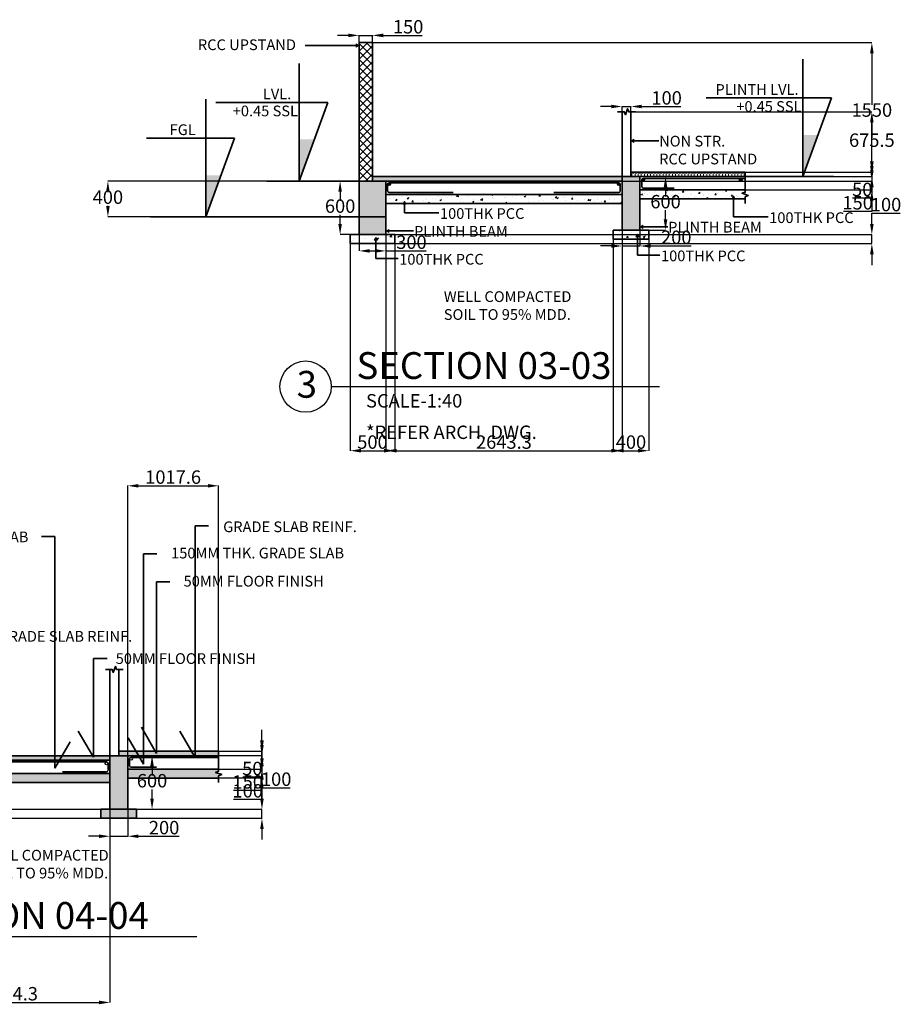
# Model space of a CAD drawing. Units: millimetres. Extents: x -174 to 32373, y 27344 to 53129.
# Tile 6 of 7: x 21438 to 31305, y 27859 to 38879. Entities that reach past the tile are written whole.
import ezdxf

# ---------------------------------------------------------------- set-up
doc = ezdxf.new("R2010")
doc.units = ezdxf.units.MM
doc.header["$LTSCALE"] = 50
for name, color, linetype, lineweight in [('S-ANNO-DIMS', 2, 'Continuous', 18), ('S-ANNO-SYMB', 4, 'Continuous', 25), ('S-ANNO-TEXT', 3, 'Continuous', 18), ('S-DETL', 7, 'Continuous', 35), ('S-PATT', 8, 'Continuous', 13), ('S-REIN', 1, 'Continuous', 25)]:
    doc.layers.add(name, color=color, linetype=linetype, lineweight=lineweight)
doc.styles.get("Standard").update_dxf_attribs({"font": 'arial.ttf'})
doc.dimstyles.new('ISO-25', dxfattribs={"dimtxt": 150, "dimasz": 120, "dimexe": 1.25, "dimexo": 0.625, "dimtad": 1, "dimtih": 1, "dimtoh": 1, "dimdec": 0, "dimtxsty": 'Standard', "dimcen": 2.5, "dimadec": 0, "dimazin": 0, "dimtfac": 1, "dimtdec": 0, "dimtmove": 0, "dimatfit": 3, "dimfxl": 1, "dimarcsym": 0})
pattern_1 = [(0, (0, 0), (0, 34.925), [25.4, -9.525]), (90, (0, 0), (-34.925, 2e-15), [25.4, -9.525])]

# ---------------------------------------------------------------- blocks, each defined once
blk = doc.blocks.new('*D20')
at = {"layer": 'Defpoints', "color": 0, "transparency": 16777216}
for p in [(28179, 36523), (28379, 36523), (28379, 36346)]:
    blk.add_point(p, dxfattribs=at)
at = {"layer": 'S-ANNO-DIMS', "color": 0, "lineweight": -2, "transparency": 16777216}
for p, q in [((28179, 36522), (28179, 36345)), ((28379, 36522), (28379, 36345)), ((28059, 36346), (27939, 36346)), ((28179, 36346), (28379, 36346)), ((28499, 36346), (28954, 36346))]:
    blk.add_line(p, q, dxfattribs=at)
at = {"layer": 'S-ANNO-DIMS', "color": 0, "transparency": 16777216}
for points in [[(28059, 36366), (28059, 36326), (28179, 36346)], [(28499, 36366), (28499, 36326), (28379, 36346)]]:
    blk.add_solid(points, dxfattribs=at)
at = {"layer": 'S-ANNO-DIMS', "color": 0, "transparency": 16777216, "insert": (28786, 36424), "char_height": 150, "attachment_point": 5}
blk.add_mtext('200', dxfattribs=at)
blk = doc.blocks.new('*D21')
at = {"layer": 'Defpoints', "color": 0, "transparency": 16777216}
for p in [(28379, 37123), (28666, 37123), (28379, 36523)]:
    blk.add_point(p, dxfattribs=at)
at = {"layer": 'S-ANNO-DIMS', "color": 0, "lineweight": -2, "transparency": 16777216}
for p, q in [((28380, 37123), (28667, 37123)), ((28666, 37003), (28666, 36900)), ((28666, 36643), (28666, 36746)), ((28380, 36523), (28667, 36523))]:
    blk.add_line(p, q, dxfattribs=at)
at = {"layer": 'S-ANNO-DIMS', "color": 0, "transparency": 16777216}
for points in [[(28646, 37003), (28686, 37003), (28666, 37123)], [(28646, 36643), (28686, 36643), (28666, 36523)]]:
    blk.add_solid(points, dxfattribs=at)
at = {"layer": 'S-ANNO-DIMS', "color": 0, "transparency": 16777216, "insert": (28666, 36823), "char_height": 150, "attachment_point": 5}
blk.add_mtext('600', dxfattribs=at)
blk = doc.blocks.new('*D22')
at = {"layer": 'Defpoints', "color": 0, "transparency": 16777216}
for p in [(25024, 37073), (25536, 37073), (25536, 36473)]:
    blk.add_point(p, dxfattribs=at)
at = {"layer": 'S-ANNO-DIMS', "color": 0, "lineweight": -2, "transparency": 16777216}
for p, q in [((25535, 37073), (25023, 37073)), ((25024, 36953), (25024, 36850)), ((25024, 36593), (25024, 36696)), ((25535, 36473), (25023, 36473))]:
    blk.add_line(p, q, dxfattribs=at)
at = {"layer": 'S-ANNO-DIMS', "color": 0, "transparency": 16777216}
for points in [[(25004, 36953), (25044, 36953), (25024, 37073)], [(25004, 36593), (25044, 36593), (25024, 36473)]]:
    blk.add_solid(points, dxfattribs=at)
at = {"layer": 'S-ANNO-DIMS', "color": 0, "transparency": 16777216, "insert": (25024, 36773), "char_height": 150, "attachment_point": 5}
blk.add_mtext('600', dxfattribs=at)
blk = doc.blocks.new('*D23')
at = {"layer": 'Defpoints', "color": 0, "transparency": 16777216}
for p in [(25236, 36473), (25536, 36473), (25536, 36291)]:
    blk.add_point(p, dxfattribs=at)
at = {"layer": 'S-ANNO-DIMS', "color": 0, "lineweight": -2, "transparency": 16777216}
for p, q in [((25236, 36472), (25236, 36290)), ((25536, 36472), (25536, 36290)), ((25356, 36291), (25416, 36291)), ((25536, 36291), (25988, 36291))]:
    blk.add_line(p, q, dxfattribs=at)
at = {"layer": 'S-ANNO-DIMS', "color": 0, "transparency": 16777216}
for points in [[(25356, 36311), (25356, 36271), (25236, 36291)], [(25416, 36311), (25416, 36271), (25536, 36291)]]:
    blk.add_solid(points, dxfattribs=at)
at = {"layer": 'S-ANNO-DIMS', "color": 0, "transparency": 16777216, "insert": (25822, 36369), "char_height": 150, "attachment_point": 5}
blk.add_mtext('300', dxfattribs=at)
blk = doc.blocks.new('*D24')
at = {"layer": 'Defpoints', "color": 0, "transparency": 16777216}
for p in [(25386, 38703), (25236, 38623), (25386, 38623)]:
    blk.add_point(p, dxfattribs=at)
at = {"layer": 'S-ANNO-DIMS', "color": 0, "lineweight": -2, "transparency": 16777216}
for p, q in [((25116, 38703), (24996, 38703)), ((25236, 38624), (25236, 38704)), ((25236, 38703), (25386, 38703)), ((25386, 38624), (25386, 38704)), ((25506, 38703), (25944, 38703))]:
    blk.add_line(p, q, dxfattribs=at)
at = {"layer": 'S-ANNO-DIMS', "color": 0, "transparency": 16777216}
for points in [[(25116, 38723), (25116, 38683), (25236, 38703)], [(25506, 38723), (25506, 38683), (25386, 38703)]]:
    blk.add_solid(points, dxfattribs=at)
at = {"layer": 'S-ANNO-DIMS', "color": 0, "transparency": 16777216, "insert": (25785, 38780), "char_height": 150, "attachment_point": 5}
blk.add_mtext('150', dxfattribs=at)
blk = doc.blocks.new('*D25')
at = {"layer": 'Defpoints', "color": 0, "transparency": 16777216}
for p in [(28179, 37849), (28279, 37907), (28279, 37849)]:
    blk.add_point(p, dxfattribs=at)
at = {"layer": 'S-ANNO-DIMS', "color": 0, "lineweight": -2, "transparency": 16777216}
for p, q in [((28179, 37849), (28179, 37908)), ((28279, 37849), (28279, 37908)), ((28059, 37907), (27939, 37907)), ((28179, 37907), (28279, 37907)), ((28399, 37907), (28837, 37907))]:
    blk.add_line(p, q, dxfattribs=at)
at = {"layer": 'S-ANNO-DIMS', "color": 0, "transparency": 16777216}
for points in [[(28059, 37927), (28059, 37887), (28179, 37907)], [(28399, 37927), (28399, 37887), (28279, 37907)]]:
    blk.add_solid(points, dxfattribs=at)
at = {"layer": 'S-ANNO-DIMS', "color": 0, "transparency": 16777216, "insert": (28678, 37984), "char_height": 150, "attachment_point": 5}
blk.add_mtext('100', dxfattribs=at)
blk = doc.blocks.new('*D27')
at = {"layer": 'Defpoints', "color": 0, "transparency": 16777216}
for p in [(22447, 30042), (22647, 30042), (22647, 29740)]:
    blk.add_point(p, dxfattribs=at)
at = {"layer": 'S-ANNO-DIMS', "color": 0, "lineweight": -2, "transparency": 16777216}
for p, q in [((22447, 30041), (22447, 29739)), ((22647, 30041), (22647, 29739)), ((22327, 29740), (22207, 29740)), ((22447, 29740), (22647, 29740)), ((22767, 29740), (23221, 29740))]:
    blk.add_line(p, q, dxfattribs=at)
at = {"layer": 'S-ANNO-DIMS', "color": 0, "transparency": 16777216}
for points in [[(22327, 29760), (22327, 29720), (22447, 29740)], [(22767, 29760), (22767, 29720), (22647, 29740)]]:
    blk.add_solid(points, dxfattribs=at)
at = {"layer": 'S-ANNO-DIMS', "color": 0, "transparency": 16777216, "insert": (23054, 29817), "char_height": 150, "attachment_point": 5}
blk.add_mtext('200', dxfattribs=at)
blk = doc.blocks.new('*D29')
at = {"layer": 'Defpoints', "color": 0, "transparency": 16777216}
for p in [(22647, 30642), (22647, 30042), (22919, 30042)]:
    blk.add_point(p, dxfattribs=at)
at = {"layer": 'S-ANNO-DIMS', "color": 0, "lineweight": -2, "transparency": 16777216}
for p, q in [((22647, 30642), (22921, 30642)), ((22919, 30522), (22919, 30419)), ((22919, 30162), (22919, 30265)), ((22647, 30042), (22921, 30042))]:
    blk.add_line(p, q, dxfattribs=at)
at = {"layer": 'S-ANNO-DIMS', "color": 0, "transparency": 16777216}
for points in [[(22899, 30522), (22939, 30522), (22919, 30642)], [(22899, 30162), (22939, 30162), (22919, 30042)]]:
    blk.add_solid(points, dxfattribs=at)
at = {"layer": 'S-ANNO-DIMS', "color": 0, "transparency": 16777216, "insert": (22919, 30342), "char_height": 150, "attachment_point": 5}
blk.add_mtext('600', dxfattribs=at)
blk = doc.blocks.new('SECTION-MARK')
blk.add_line((575, 287), (4248, 287))
blk.add_circle((287, 287), 287)
blk = doc.blocks.new('*D76')
at = {"layer": 'Defpoints', "color": 0, "transparency": 16777216}
for p in [(22425, 37073), (25236, 37073), (25536, 36673)]:
    blk.add_point(p, dxfattribs=at)
at = {"layer": 'S-ANNO-DIMS', "color": 0, "lineweight": -2, "transparency": 16777216}
for p, q in [((25235, 37073), (22424, 37073)), ((22425, 36953), (22425, 36950)), ((22425, 36793), (22425, 36796)), ((25535, 36673), (22424, 36673))]:
    blk.add_line(p, q, dxfattribs=at)
at = {"layer": 'S-ANNO-DIMS', "color": 0, "transparency": 16777216}
for points in [[(22405, 36953), (22445, 36953), (22425, 37073)], [(22405, 36793), (22445, 36793), (22425, 36673)]]:
    blk.add_solid(points, dxfattribs=at)
at = {"layer": 'S-ANNO-DIMS', "color": 0, "transparency": 16777216, "insert": (22425, 36873), "char_height": 150, "attachment_point": 5}
blk.add_mtext('400', dxfattribs=at)
blk = doc.blocks.new('*D77')
at = {"layer": 'Defpoints', "color": 0, "transparency": 16777216}
for p in [(25386, 38623), (30975, 38623), (25386, 37073)]:
    blk.add_point(p, dxfattribs=at)
at = {"layer": 'S-ANNO-DIMS', "color": 0, "lineweight": -2, "transparency": 16777216}
for p, q in [((25386, 38623), (30976, 38623)), ((30975, 38503), (30975, 37925)), ((30975, 37193), (30975, 37771)), ((25386, 37073), (30976, 37073))]:
    blk.add_line(p, q, dxfattribs=at)
at = {"layer": 'S-ANNO-DIMS', "color": 0, "transparency": 16777216}
for points in [[(30955, 38503), (30995, 38503), (30975, 38623)], [(30955, 37193), (30995, 37193), (30975, 37073)]]:
    blk.add_solid(points, dxfattribs=at)
at = {"layer": 'S-ANNO-DIMS', "color": 0, "transparency": 16777216, "insert": (30975, 37848), "char_height": 150, "attachment_point": 5}
blk.add_mtext('1550', dxfattribs=at)
blk = doc.blocks.new('*D78')
at = {"layer": 'Defpoints', "color": 0, "transparency": 16777216}
for p in [(28179, 36523), (25536, 36473), (28179, 34055)]:
    blk.add_point(p, dxfattribs=at)
at = {"layer": 'S-ANNO-DIMS', "color": 0, "lineweight": -2, "transparency": 16777216}
for p, q in [((28179, 36522), (28179, 34054)), ((25536, 36472), (25536, 34054)), ((25656, 34055), (28059, 34055))]:
    blk.add_line(p, q, dxfattribs=at)
at = {"layer": 'S-ANNO-DIMS', "color": 0, "transparency": 16777216}
for points in [[(25656, 34075), (25656, 34035), (25536, 34055)], [(28059, 34075), (28059, 34035), (28179, 34055)]]:
    blk.add_solid(points, dxfattribs=at)
at = {"layer": 'S-ANNO-DIMS', "color": 0, "transparency": 16777216, "insert": (26857, 34132), "char_height": 150, "attachment_point": 5}
blk.add_mtext('2643.3', dxfattribs=at)
blk = doc.blocks.new('*D79')
at = {"layer": 'Defpoints', "color": 0, "transparency": 16777216}
for p in [(29557, 37173), (28379, 37123), (30975, 37123)]:
    blk.add_point(p, dxfattribs=at)
at = {"layer": 'S-ANNO-DIMS', "color": 0, "lineweight": -2, "transparency": 16777216}
for p, q in [((30975, 37293), (30975, 37413)), ((29558, 37173), (30976, 37173)), ((30975, 37173), (30975, 37123)), ((28380, 37123), (30976, 37123)), ((30975, 37003), (30975, 36883)), ((30975, 36883), (30760, 36883))]:
    blk.add_line(p, q, dxfattribs=at)
at = {"layer": 'S-ANNO-DIMS', "color": 0, "transparency": 16777216}
for points in [[(30955, 37293), (30995, 37293), (30975, 37173)], [(30955, 37003), (30995, 37003), (30975, 37123)]]:
    blk.add_solid(points, dxfattribs=at)
at = {"layer": 'S-ANNO-DIMS', "color": 0, "transparency": 16777216, "insert": (30867, 36960), "char_height": 150, "attachment_point": 5}
blk.add_mtext('50', dxfattribs=at)
blk = doc.blocks.new('*D80')
at = {"layer": 'Defpoints', "color": 0, "transparency": 16777216}
for p in [(28379, 37123), (29557, 36973), (30975, 36973)]:
    blk.add_point(p, dxfattribs=at)
at = {"layer": 'S-ANNO-DIMS', "color": 0, "lineweight": -2, "transparency": 16777216}
for p, q in [((30975, 37243), (30975, 37363)), ((28380, 37123), (30976, 37123)), ((30975, 37123), (30975, 36973)), ((29558, 36973), (30976, 36973)), ((30975, 36853), (30975, 36733)), ((30975, 36733), (30658, 36733))]:
    blk.add_line(p, q, dxfattribs=at)
at = {"layer": 'S-ANNO-DIMS', "color": 0, "transparency": 16777216}
for points in [[(30955, 37243), (30995, 37243), (30975, 37123)], [(30955, 36853), (30995, 36853), (30975, 36973)]]:
    blk.add_solid(points, dxfattribs=at)
at = {"layer": 'S-ANNO-DIMS', "color": 0, "transparency": 16777216, "insert": (30816, 36810), "char_height": 150, "attachment_point": 5}
blk.add_mtext('150', dxfattribs=at)
blk = doc.blocks.new('*D81')
at = {"layer": 'Defpoints', "color": 0, "transparency": 16777216}
for p in [(28279, 37849), (30975, 37849), (28279, 37173)]:
    blk.add_point(p, dxfattribs=at)
at = {"layer": 'S-ANNO-DIMS', "color": 0, "lineweight": -2, "transparency": 16777216}
for p, q in [((28280, 37849), (30976, 37849)), ((30975, 37729), (30975, 37588)), ((30975, 37293), (30975, 37434)), ((28280, 37173), (30976, 37173))]:
    blk.add_line(p, q, dxfattribs=at)
at = {"layer": 'S-ANNO-DIMS', "color": 0, "transparency": 16777216}
for points in [[(30955, 37729), (30995, 37729), (30975, 37849)], [(30955, 37293), (30995, 37293), (30975, 37173)]]:
    blk.add_solid(points, dxfattribs=at)
at = {"layer": 'S-ANNO-DIMS', "color": 0, "transparency": 16777216, "insert": (30975, 37511), "char_height": 150, "attachment_point": 5}
blk.add_mtext('675.5', dxfattribs=at)
blk = doc.blocks.new('*D82')
at = {"layer": 'Defpoints', "color": 0, "transparency": 16777216}
for p in [(25136, 36373), (25636, 36373), (25636, 34055)]:
    blk.add_point(p, dxfattribs=at)
at = {"layer": 'S-ANNO-DIMS', "color": 0, "lineweight": -2, "transparency": 16777216}
for p, q in [((25136, 36372), (25136, 34054)), ((25636, 36372), (25636, 34054)), ((25256, 34055), (25516, 34055))]:
    blk.add_line(p, q, dxfattribs=at)
at = {"layer": 'S-ANNO-DIMS', "color": 0, "transparency": 16777216}
for points in [[(25256, 34075), (25256, 34035), (25136, 34055)], [(25516, 34075), (25516, 34035), (25636, 34055)]]:
    blk.add_solid(points, dxfattribs=at)
at = {"layer": 'S-ANNO-DIMS', "color": 0, "transparency": 16777216, "insert": (25386, 34132), "char_height": 150, "attachment_point": 5}
blk.add_mtext('500', dxfattribs=at)
blk = doc.blocks.new('*D83')
at = {"layer": 'Defpoints', "color": 0, "transparency": 16777216}
for p in [(28079, 36423), (28479, 36423), (28479, 34055)]:
    blk.add_point(p, dxfattribs=at)
at = {"layer": 'S-ANNO-DIMS', "color": 0, "lineweight": -2, "transparency": 16777216}
for p, q in [((28079, 36422), (28079, 34054)), ((28479, 36422), (28479, 34054)), ((28199, 34055), (28359, 34055))]:
    blk.add_line(p, q, dxfattribs=at)
at = {"layer": 'S-ANNO-DIMS', "color": 0, "transparency": 16777216}
for points in [[(28199, 34075), (28199, 34035), (28079, 34055)], [(28359, 34075), (28359, 34035), (28479, 34055)]]:
    blk.add_solid(points, dxfattribs=at)
at = {"layer": 'S-ANNO-DIMS', "color": 0, "transparency": 16777216, "insert": (28279, 34132), "char_height": 150, "attachment_point": 5}
blk.add_mtext('400', dxfattribs=at)
blk = doc.blocks.new('*D84')
at = {"layer": 'Defpoints', "color": 0, "transparency": 16777216}
for p in [(25636, 36473), (25636, 36373), (30975, 36473)]:
    blk.add_point(p, dxfattribs=at)
at = {"layer": 'S-ANNO-DIMS', "color": 0, "lineweight": -2, "transparency": 16777216}
for p, q in [((30975, 36593), (30975, 36713)), ((30975, 36713), (31293, 36713)), ((25636, 36473), (30976, 36473)), ((25636, 36373), (30976, 36373)), ((30975, 36373), (30975, 36473)), ((30975, 36253), (30975, 36133))]:
    blk.add_line(p, q, dxfattribs=at)
at = {"layer": 'S-ANNO-DIMS', "color": 0, "transparency": 16777216}
for points in [[(30955, 36593), (30995, 36593), (30975, 36473)], [(30955, 36253), (30995, 36253), (30975, 36373)]]:
    blk.add_solid(points, dxfattribs=at)
at = {"layer": 'S-ANNO-DIMS', "color": 0, "transparency": 16777216, "insert": (31134, 36790), "char_height": 150, "attachment_point": 5}
blk.add_mtext('100', dxfattribs=at)
blk = doc.blocks.new('*D85')
at = {"layer": 'Defpoints', "color": 0, "transparency": 16777216}
for p in [(20212, 30042), (22447, 30042), (22447, 27880)]:
    blk.add_point(p, dxfattribs=at)
at = {"layer": 'S-ANNO-DIMS', "color": 0, "lineweight": -2, "transparency": 16777216}
for p, q in [((20212, 30041), (20212, 27879)), ((22447, 30041), (22447, 27879)), ((20332, 27880), (22327, 27880))]:
    blk.add_line(p, q, dxfattribs=at)
at = {"layer": 'S-ANNO-DIMS', "color": 0, "transparency": 16777216}
for points in [[(20332, 27900), (20332, 27860), (20212, 27880)], [(22327, 27900), (22327, 27860), (22447, 27880)]]:
    blk.add_solid(points, dxfattribs=at)
at = {"layer": 'S-ANNO-DIMS', "color": 0, "transparency": 16777216, "insert": (21330, 27958), "char_height": 150, "attachment_point": 5}
blk.add_mtext('2234.3', dxfattribs=at)
blk = doc.blocks.new('*D86')
at = {"layer": 'Defpoints', "color": 0, "transparency": 16777216}
for p in [(22647, 30642), (23664, 30692), (24149, 30642)]:
    blk.add_point(p, dxfattribs=at)
at = {"layer": 'S-ANNO-DIMS', "color": 0, "lineweight": -2, "transparency": 16777216}
for p, q in [((24149, 30812), (24149, 30932)), ((22647, 30642), (24150, 30642)), ((23665, 30692), (24150, 30692)), ((24149, 30692), (24149, 30642)), ((24149, 30522), (24149, 30402)), ((24149, 30402), (23934, 30402))]:
    blk.add_line(p, q, dxfattribs=at)
at = {"layer": 'S-ANNO-DIMS', "color": 0, "transparency": 16777216}
for points in [[(24129, 30812), (24169, 30812), (24149, 30692)], [(24129, 30522), (24169, 30522), (24149, 30642)]]:
    blk.add_solid(points, dxfattribs=at)
at = {"layer": 'S-ANNO-DIMS', "color": 0, "transparency": 16777216, "insert": (24041, 30479), "char_height": 150, "attachment_point": 5}
blk.add_mtext('50', dxfattribs=at)
blk = doc.blocks.new('*D87')
at = {"layer": 'Defpoints', "color": 0, "transparency": 16777216}
for p in [(22647, 30642), (23664, 30492), (24149, 30492)]:
    blk.add_point(p, dxfattribs=at)
at = {"layer": 'S-ANNO-DIMS', "color": 0, "lineweight": -2, "transparency": 16777216}
for p, q in [((24149, 30762), (24149, 30882)), ((22647, 30642), (24150, 30642)), ((24149, 30642), (24149, 30492)), ((23665, 30492), (24150, 30492)), ((24149, 30372), (24149, 30252)), ((24149, 30252), (23831, 30252))]:
    blk.add_line(p, q, dxfattribs=at)
at = {"layer": 'S-ANNO-DIMS', "color": 0, "transparency": 16777216}
for points in [[(24129, 30762), (24169, 30762), (24149, 30642)], [(24129, 30372), (24169, 30372), (24149, 30492)]]:
    blk.add_solid(points, dxfattribs=at)
at = {"layer": 'S-ANNO-DIMS', "color": 0, "transparency": 16777216, "insert": (23990, 30329), "char_height": 150, "attachment_point": 5}
blk.add_mtext('150', dxfattribs=at)
blk = doc.blocks.new('*D88')
at = {"layer": 'Defpoints', "color": 0, "transparency": 16777216}
for p in [(23664, 30492), (23664, 30392), (24149, 30392)]:
    blk.add_point(p, dxfattribs=at)
at = {"layer": 'S-ANNO-DIMS', "color": 0, "lineweight": -2, "transparency": 16777216}
for p, q in [((24149, 30612), (24149, 30732)), ((23665, 30492), (24150, 30492)), ((24149, 30492), (24149, 30392)), ((23665, 30392), (24150, 30392)), ((24149, 30272), (24149, 30152)), ((24149, 30152), (23831, 30152))]:
    blk.add_line(p, q, dxfattribs=at)
at = {"layer": 'S-ANNO-DIMS', "color": 0, "transparency": 16777216}
for points in [[(24129, 30612), (24169, 30612), (24149, 30492)], [(24129, 30272), (24169, 30272), (24149, 30392)]]:
    blk.add_solid(points, dxfattribs=at)
at = {"layer": 'S-ANNO-DIMS', "color": 0, "transparency": 16777216, "insert": (23990, 30229), "char_height": 150, "attachment_point": 5}
blk.add_mtext('100', dxfattribs=at)
blk = doc.blocks.new('*D90')
at = {"layer": 'Defpoints', "color": 0, "transparency": 16777216}
for p in [(23664, 33662), (22647, 30642), (23664, 30692)]:
    blk.add_point(p, dxfattribs=at)
at = {"layer": 'S-ANNO-DIMS', "color": 0, "lineweight": -2, "transparency": 16777216}
for p, q in [((22647, 30642), (22647, 33664)), ((22767, 33662), (23544, 33662)), ((23664, 30692), (23664, 33664))]:
    blk.add_line(p, q, dxfattribs=at)
at = {"layer": 'S-ANNO-DIMS', "color": 0, "transparency": 16777216}
for points in [[(22767, 33682), (22767, 33642), (22647, 33662)], [(23544, 33682), (23544, 33642), (23664, 33662)]]:
    blk.add_solid(points, dxfattribs=at)
at = {"layer": 'S-ANNO-DIMS', "color": 0, "transparency": 16777216, "insert": (23155, 33740), "char_height": 150, "attachment_point": 5}
blk.add_mtext('1017.6', dxfattribs=at)
blk = doc.blocks.new('*D92')
at = {"layer": 'Defpoints', "color": 0, "transparency": 16777216}
for p in [(20312, 30042), (24149, 30042), (20312, 29942)]:
    blk.add_point(p, dxfattribs=at)
at = {"layer": 'S-ANNO-DIMS', "color": 0, "lineweight": -2, "transparency": 16777216}
for p, q in [((24149, 30162), (24149, 30282)), ((24149, 30282), (24466, 30282)), ((20313, 30042), (24150, 30042)), ((24149, 29942), (24149, 30042)), ((20313, 29942), (24150, 29942)), ((24149, 29822), (24149, 29702))]:
    blk.add_line(p, q, dxfattribs=at)
at = {"layer": 'S-ANNO-DIMS', "color": 0, "transparency": 16777216}
for points in [[(24129, 30162), (24169, 30162), (24149, 30042)], [(24129, 29822), (24169, 29822), (24149, 29942)]]:
    blk.add_solid(points, dxfattribs=at)
at = {"layer": 'S-ANNO-DIMS', "color": 0, "transparency": 16777216, "insert": (24308, 30359), "char_height": 150, "attachment_point": 5}
blk.add_mtext('100', dxfattribs=at)

msp = doc.modelspace()

# ---------------------------------------------------------------- hatches: boundary and pattern name
at = {"layer": 'S-ANNO-SYMB'}
h = msp.add_hatch(color=256, dxfattribs=at)
h.dxf.hatch_style = 1
h.paths.add_polyline_path([(30201.87, 37123.04), (30371.08, 37587.96), (30201.87, 37587.96)])
h = msp.add_hatch(color=256, dxfattribs=at)
h.dxf.hatch_style = 1
h.paths.add_polyline_path([(24566.02, 37073.04), (24735.24, 37537.96), (24566.02, 37537.96)])
h = msp.add_hatch(color=256, dxfattribs=at)
h.dxf.hatch_style = 1
h.paths.add_polyline_path([(23522.69, 36673.04), (23691.91, 37137.96), (23522.69, 37137.96)])
at = {"layer": 'S-ANNO-TEXT'}
h = msp.add_hatch(color=256, dxfattribs=at)
h.dxf.hatch_style = 1
h.paths.add_polyline_path([(25204.09, 38607.16), (25204.09, 38570.5), (25235.84, 38588.83)])
h = msp.add_hatch(color=256, dxfattribs=at)
h.dxf.hatch_style = 1
h.paths.add_polyline_path([(28279.14, 37523.37), (28310.89, 37505.04), (28310.89, 37541.71)])
h = msp.add_hatch(color=256, dxfattribs=at)
h.dxf.hatch_style = 1
h.paths.add_polyline_path([(25571.7, 37053.04, 0.40886497), (25555.84, 37037.19, 0.99539446), (25587.26, 37037.33, 0.41151206)])
h = msp.add_hatch(color=256, dxfattribs=at)
h.dxf.hatch_style = 1
h.paths.add_polyline_path([(28159.14, 37037.33, 1), (28127.72, 37037.33, 1)])
h = msp.add_hatch(color=256, dxfattribs=at)
h.dxf.hatch_style = 1
h.paths.add_polyline_path([(28430.56, 37087.33, 1), (28399.14, 37087.33, 1)])
h = msp.add_hatch(color=256, dxfattribs=at)
h.dxf.hatch_style = 1
h.paths.add_polyline_path([(29522.57, 37087.33, 1), (29491.15, 37087.33, 1)])
h = msp.add_hatch(color=256, dxfattribs=at)
h.dxf.hatch_style = 1
h.paths.add_polyline_path([(25743.42, 36845.8), (25725.08, 36814.04), (25761.75, 36814.04)])
h = msp.add_hatch(color=256, dxfattribs=at)
h.dxf.hatch_style = 1
h.paths.add_polyline_path([(29427.68, 36907.17), (29409.34, 36875.42), (29446.01, 36875.42)])
h = msp.add_hatch(color=256, dxfattribs=at)
h.dxf.hatch_style = 1
h.paths.add_polyline_path([(25535.84, 36513.92), (25567.6, 36495.59), (25567.6, 36532.25)])
h = msp.add_hatch(color=256, dxfattribs=at)
h.dxf.hatch_style = 1
h.paths.add_polyline_path([(28352.38, 36479.44), (28334.05, 36447.69), (28370.71, 36447.69)])
h = msp.add_hatch(color=256, dxfattribs=at)
h.dxf.hatch_style = 1
h.paths.add_polyline_path([(28379.14, 36560.36), (28410.89, 36542.03), (28410.89, 36578.69)])
h = msp.add_hatch(color=256, dxfattribs=at)
h.dxf.hatch_style = 1
h.paths.add_polyline_path([(25422.3, 36441.56), (25403.97, 36409.81), (25440.63, 36409.81)])
at = {"layer": 'S-PATT'}
h = msp.add_hatch(dxfattribs=at)
h.set_pattern_fill('ANSI37', color=256, scale=20)
h.paths.add_polyline_path([(25235.84, 37073.04), (25385.84, 37073.04), (25385.84, 38623.04), (25235.84, 38623.04)])
h = msp.add_hatch(dxfattribs=at)
h.set_pattern_fill('ANGLE', color=256, scale=5)
h.set_pattern_definition(pattern_1)
h.paths.add_polyline_path([(29557.2, 37123.04), (29557.2, 37173.04), (28279.14, 37173.04), (28279.14, 37123.04), (28379.14, 37123.04)])
h = msp.add_hatch(color=256, dxfattribs=at)
h.dxf.hatch_style = 1
h.paths.add_polyline_path([(25535.84, 37073.04), (25235.84, 37073.04), (25235.84, 36473.04), (25535.84, 36473.04)])
h = msp.add_hatch(dxfattribs=at)
h.set_pattern_fill('ANGLE', color=256, scale=5)
h.set_pattern_definition(pattern_1)
h.paths.add_polyline_path([(28179.14, 37073.04), (28179.14, 37123.04), (25385.84, 37123.04), (25385.84, 37073.04), (25535.84, 37073.04)])
h = msp.add_hatch(color=256, dxfattribs=at)
h.dxf.hatch_style = 1
h.paths.add_polyline_path([(28179.14, 36523.04), (28379.14, 36523.04), (28379.14, 37123.04), (28179.14, 37123.04)])
h = msp.add_hatch(dxfattribs=at)
h.set_pattern_fill('AR-CONC', color=256)
h.paths.add_polyline_path([(28179.14, 36923.04), (25535.84, 36923.04), (25535.84, 36823.04), (28179.14, 36823.04)])
h = msp.add_hatch(dxfattribs=at)
h.set_pattern_fill('AR-CONC', color=256)
h.paths.add_polyline_path([(28379.14, 36973.04), (28379.14, 36873.04), (29557.2, 36873.04), (29557.2, 36898.04), (29591.54, 36910.54), (29522.86, 36935.54), (29557.2, 36948.04), (29557.2, 36973.04)])
h = msp.add_hatch(dxfattribs=at)
h.set_pattern_fill('AR-CONC', color=256)
h.paths.add_polyline_path([(28479.14, 36523.04), (28379.14, 36523.04), (28179.14, 36523.04), (28079.14, 36523.04), (28079.14, 36423.04), (28479.14, 36423.04)])
h = msp.add_hatch(dxfattribs=at)
h.set_pattern_fill('AR-CONC', color=256)
h.paths.add_polyline_path([(25635.84, 36473.04), (25535.84, 36473.04), (25235.84, 36473.04), (25135.84, 36473.04), (25135.84, 36373.04), (25635.84, 36373.04)])
h = msp.add_hatch(dxfattribs=at)
h.set_pattern_fill('ANGLE', color=256, scale=5)
h.set_pattern_definition([(0, (-5178.336, 733.413), (0, 34.925), [25.4, -9.525]), (90, (-5178.336, 733.413), (-34.925, 2e-15), [25.4, -9.525])])
h.paths.add_polyline_path([(22446.68, 30591.75), (22446.68, 30641.75), (20212.39, 30641.75), (20212.39, 30591.75)])
h.paths.add_polyline_path([(20012.39, 30641.75), (20112.39, 30641.75), (20112.39, 30691.75), (19005.68, 30691.75), (19005.68, 30641.75)])
h.paths.add_polyline_path([(22546.68, 30691.75), (22546.68, 30641.75), (22646.68, 30641.75), (23664.24, 30641.75), (23664.24, 30691.75)])
h = msp.add_hatch(color=256, dxfattribs=at)
h.dxf.hatch_style = 1
h.paths.add_polyline_path([(20212.39, 30641.75), (20012.39, 30641.75), (20012.39, 30041.75), (20212.39, 30041.75)])
h.paths.add_polyline_path([(22646.68, 30641.75), (22446.68, 30641.75), (22446.68, 30041.75), (22646.68, 30041.75)])
h = msp.add_hatch(dxfattribs=at)
h.set_pattern_fill('AR-CONC', color=256)
h.set_pattern_definition([(50, (-5178.34, 733.41), (182.18467, -15.9391), [19.05, -209.55]), (355, (-5178.34, 733.41), (-35.2434, 191.05685), [15.24, -167.6406]), (100.45144, (-5163.15, 732.09), (146.94125, 175.11775), [16.19, -178.09024]), (46.1842, (-5178.34, 784.21), (271.079, -42.0423), [28.575, -314.325]), (96.63556, (-5155.75, 780.7), (237.4041, 247.4261), [24.285, -267.1356]), (351.18415, (-5178.34, 784.2), (237.4041, 247.4261), [22.86, -251.4597]), (21, (-5152.94, 771.51), (151.6144, -102.2652), [19.05, -209.55]), (326, (-5152.94, 771.51), (61.802, 184.188), [15.24, -167.64]), (71.45144, (-5140.3, 762.99), (213.4164, 81.9228), [16.19, -178.0899]), (37.5, (-5178.336, 733.413), (3.0886, 84.55504), [0, -165.608, 0, -170.18, 0, -168.275]), (7.5, (-5178.34, 733.41), (66.81966, 100.18057), [0, -97.028, 0, -161.798, 0, -64.135]), (327.5, (-5234.98, 733.41), (135.5906, -5.72874), [0, -63.5, 0, -198.12, 0, -262.89]), (317.5, (-5260.38, 733.41), (148.12918, 25.4265), [0, -82.55, 0, -131.572, 0, -186.69])])
h.paths.add_polyline_path([(20312.39, 29941.75), (20312.39, 30041.75), (20212.39, 30041.75), (20012.39, 30041.75), (19912.39, 30041.75), (19912.39, 29941.75)])
h.paths.add_polyline_path([(22746.68, 29941.75), (22746.68, 30041.75), (22646.68, 30041.75), (22446.68, 30041.75), (22346.68, 30041.75), (22346.68, 29941.75)])
h.paths.add_polyline_path([(22446.68, 30341.75), (22446.68, 30441.75), (20212.39, 30441.75), (20212.39, 30341.75)])
h.paths.add_polyline_path([(23664.24, 30391.75), (23664.24, 30441.75), (23629.9, 30454.25), (23664.24, 30466.75), (23664.24, 30491.75), (22646.68, 30491.75), (22646.68, 30391.75)])
h.paths.add_polyline_path([(20012.39, 30391.75), (20012.39, 30491.75), (19005.68, 30491.75), (19005.68, 30441.75), (19040.02, 30429.25), (19005.68, 30416.75), (19005.68, 30391.75)])

# ---------------------------------------------------------------- linework, layer by layer
at = {"layer": 'S-ANNO-TEXT'}
for points in [[(25235.84, 38588.83), (25204.09, 38570.5), (25204.09, 38607.16)], [(28279.14, 37523.37), (28310.89, 37505.04), (28310.89, 37541.71)], [(25743.42, 36845.8), (25725.08, 36814.04), (25761.75, 36814.04)], [(29427.68, 36907.17), (29409.34, 36875.42), (29446.01, 36875.42)], [(25535.84, 36513.92), (25567.6, 36495.59), (25567.6, 36532.25)], [(28352.38, 36479.44), (28334.05, 36447.69), (28370.71, 36447.69)], [(28379.14, 36560.36), (28410.89, 36542.03), (28410.89, 36578.69)], [(25422.3, 36441.56), (25403.97, 36409.81), (25440.63, 36409.81)]]:
    msp.add_lwpolyline(points, close=True, dxfattribs=at)
at = {"layer": 'S-DETL'}
for p, q in [((25204.09, 38588.83), (24631.33, 38588.83)), ((25235.84, 38623.04), (25235.84, 37073.04)), ((25235.84, 38623.04), (25385.84, 38623.04)), ((25385.84, 38623.04), (25385.84, 37073.04)), ((24566.02, 37073.04), (24566.02, 38388.54)), ((30201.87, 37123.04), (30201.87, 38438.54)), ((23522.69, 36673.04), (23522.69, 37988.54)), ((24886.09, 37952.42), (23633.71, 37952.42)), ((24566.02, 37073.04), (24886.09, 37952.42)), ((30521.93, 38002.42), (29121.86, 38002.42)), ((30201.87, 37123.04), (30521.93, 38002.42)), ((28179.14, 37123.04), (28179.14, 37848.58)), ((28279.14, 37123.04), (28279.14, 37848.58)), ((23842.76, 37552.42), (22855.16, 37552.42)), ((23522.69, 36673.04), (23842.76, 37552.42)), ((28310.89, 37523.37), (28590.28, 37523.37)), ((28279.14, 37173.04), (29557.2, 37173.04)), ((29557.2, 37023.04), (29557.2, 37173.04)), ((25535.84, 37073.04), (24201.98, 37073.04)), ((25235.84, 37073.04), (25235.84, 36473.04)), ((28179.14, 37123.04), (25385.84, 37123.04)), ((28179.14, 37073.04), (25535.84, 37073.04)), ((25535.84, 36473.04), (25535.84, 37073.04)), ((25555.84, 36959.04), (25555.84, 37037.04)), ((28143.14, 37053.04), (25571.84, 37053.04)), ((28159.14, 36959.04), (28159.14, 37037.04)), ((28179.14, 37123.04), (28379.14, 37123.04)), ((28179.14, 36523.04), (28179.14, 37123.04)), ((28379.14, 37123.04), (28379.14, 36523.04)), ((28379.14, 37123.04), (30545.25, 37123.04)), ((28399.14, 37087.04), (28399.14, 37009.04)), ((28415.14, 37103.04), (29557.2, 37103.04)), ((28179.14, 36923.04), (25535.84, 36923.04)), ((26287.99, 36943.04), (25571.84, 36943.04)), ((28143.14, 36943.04), (27415.25, 36943.04)), ((28379.14, 36973.04), (29557.2, 36973.04)), ((28415.14, 36993.04), (28761.4, 36993.04)), ((28179.14, 36823.04), (25535.84, 36823.04)), ((25743.42, 36814.04), (25743.42, 36716.53)), ((28379.14, 36873.04), (29557.2, 36873.04)), ((29427.68, 36875.42), (29427.68, 36670.52)), ((25743.42, 36716.53), (26128.56, 36716.53)), ((25535.84, 36673.04), (22901.76, 36673.04)), ((29427.68, 36670.52), (29812.82, 36670.52)), ((25567.6, 36513.92), (25846.98, 36513.92)), ((28079.14, 36423.04), (28079.14, 36523.04)), ((28079.14, 36523.04), (28179.14, 36523.04)), ((28379.14, 36523.04), (28179.14, 36523.04)), ((28379.14, 36523.04), (28479.14, 36523.04)), ((28410.89, 36560.36), (28690.28, 36560.36)), ((28479.14, 36523.04), (28479.14, 36423.04)), ((25135.84, 36373.04), (25135.84, 36473.04)), ((25135.84, 36473.04), (25235.84, 36473.04)), ((25635.84, 36373.04), (25135.84, 36373.04)), ((25235.84, 36473.04), (25535.84, 36473.04)), ((25422.3, 36409.81), (25422.3, 36204.9)), ((25535.84, 36473.04), (25635.84, 36473.04)), ((25635.84, 36473.04), (25635.84, 36373.04)), ((28479.14, 36423.04), (28079.14, 36423.04)), ((28352.38, 36447.69), (28352.38, 36242.79)), ((25422.3, 36204.9), (25672.31, 36204.9)), ((28352.38, 36242.79), (28602.39, 36242.79)), ((23400.14, 30621.75), (23400.14, 33212.37)), ((23400.14, 33212.37), (23550.45, 33212.37)), ((21831.64, 33093.15), (21681.33, 33093.15)), ((21831.64, 30502.53), (21831.64, 33093.15)), ((22822.41, 30548.08), (22822.41, 32901)), ((22822.41, 32901), (22972.72, 32901)), ((22969.54, 30667.42), (22969.54, 32585.77)), ((22969.54, 32585.77), (23119.85, 32585.77)), ((22263.68, 30623.34), (22263.68, 31727.65)), ((22263.68, 31727.65), (22415.84, 31727.65)), ((22446.68, 30641.75), (22446.68, 31607.24)), ((22546.68, 30641.75), (22546.68, 31607.24)), ((22263.68, 30623.34), (22093.67, 30917.81)), ((22969.54, 30667.42), (22799.53, 30961.89)), ((23400.14, 30621.75), (23230.12, 30916.22)), ((21831.64, 30502.53), (22001.66, 30797)), ((22822.41, 30548.08), (22652.4, 30842.55)), ((20212.39, 30641.75), (22446.68, 30641.75)), ((22446.68, 30641.75), (22646.68, 30641.75)), ((22446.68, 30041.75), (22446.68, 30641.75)), ((22546.68, 30641.75), (22546.68, 30691.75)), ((22546.68, 30691.75), (23664.24, 30691.75)), ((22646.68, 30641.75), (22646.68, 30041.75)), ((22646.68, 30641.75), (23664.24, 30641.75)), ((23664.24, 30691.75), (23664.24, 30491.75)), ((20212.39, 30591.75), (22446.68, 30591.75)), ((20248.39, 30571.75), (22410.68, 30571.75)), ((22426.68, 30477.75), (22426.68, 30555.75)), ((22666.68, 30605.75), (22666.68, 30527.75)), ((22682.68, 30621.75), (23664.24, 30621.75)), ((20212.39, 30441.75), (22446.68, 30441.75)), ((21918.54, 30461.75), (22410.68, 30461.75)), ((22646.68, 30491.75), (23664.24, 30491.75)), ((22682.68, 30511.75), (22968.77, 30511.75)), ((20212.39, 30341.75), (22446.68, 30341.75)), ((22646.68, 30391.75), (23664.24, 30391.75)), ((22346.68, 29941.75), (22346.68, 30041.75)), ((22346.68, 30041.75), (22446.68, 30041.75)), ((22646.68, 30041.75), (22446.68, 30041.75)), ((22646.68, 30041.75), (22746.68, 30041.75)), ((22746.68, 30041.75), (22746.68, 29941.75)), ((22746.68, 29941.75), (22346.68, 29941.75))]:
    msp.add_line(p, q, dxfattribs=at)
for points in [[(28129.14, 37848.58), (28204.14, 37848.58), (28216.64, 37814.24), (28241.64, 37882.93), (28254.14, 37848.58), (28329.14, 37848.58)], [(29557.2, 37023.04), (29557.2, 36948.04), (29522.86, 36935.54), (29591.54, 36910.54), (29557.2, 36898.04), (29557.2, 36823.04)], [(22396.68, 31607.24), (22471.68, 31607.24), (22484.18, 31572.9), (22509.18, 31641.59), (22521.68, 31607.24), (22596.68, 31607.24)], [(23664.24, 30541.75), (23664.24, 30466.75), (23629.9, 30454.25), (23698.59, 30429.25), (23664.24, 30416.75), (23664.24, 30341.75)]]:
    msp.add_lwpolyline(points, dxfattribs=at)
at = {"layer": 'S-REIN'}
for centre, radius in [((25571.55, 37037.33), 15.71), ((28143.43, 37037.33), 15.71), ((28414.85, 37087.33), 15.71), ((29506.86, 37087.33), 15.71), ((22410.68, 30555.75), 16), ((22682.68, 30605.75), 16)]:
    msp.add_circle(centre, radius, dxfattribs=at)
for centre, start, end in [((25571.84, 37037.04), 90, 180), ((28143.72, 37037.04), 90, 180), ((28143.14, 37037.04), 0, 90), ((28415.14, 37087.04), 90, 180), ((25571.84, 36959.04), 180, 270), ((28143.14, 36959.04), 270, 0), ((28415.14, 37009.04), 180, 270), ((22410.68, 30555.75), 0, 90), ((22682.68, 30605.75), 90, 180), ((22682.68, 30527.75), 180, 270), ((22410.68, 30477.75), 270, 0)]:
    msp.add_arc(centre, 16, start, end, dxfattribs=at)

# ---------------------------------------------------------------- block references
at = {"layer": 'S-ANNO-SYMB'}
for p in [(24350.96, 34484.92), (19172.63, 28330.26)]:
    msp.add_blockref('SECTION-MARK', p, dxfattribs=at)

# ---------------------------------------------------------------- texts
at = {"layer": 'S-ANNO-TEXT'}
for s, width, insert, char_height, attachment_point in [('RCC UPSTAND', 1913.0414, (23432.54, 38658.23), 120, 1), ('PLINTH LVL.', 1913.0414, (29224.46, 38157.56), 120, 1), ('LVL.', 1913.0414, (24159.5, 38107.56), 120, 1), ('+0.45 SSL', 1913.0414, (24552.09, 37917.38), 120, 3), ('+0.45 SSL', 1913.0414, (30187.93, 37967.38), 120, 3), ('FGL', 1913.0414, (23116.17, 37707.56), 120, 1), ('NON STR.\\PRCC UPSTAND', 1913.0414, (28594.83, 37579.46), 120, 1), ('100THK PCC', 1913.0414, (26141.75, 36769.04), 120, 1), ('100THK PCC', 1913.0414, (29826.01, 36723.03), 120, 1), ('PLINTH BEAM', 1913.0414, (28694.83, 36616.44), 120, 1), ('PLINTH BEAM', 1913.0414, (25851.54, 36570), 120, 1), ('100THK PCC', 1913.0414, (25685.5, 36257.42), 120, 1), ('100THK PCC', 1913.0414, (28615.58, 36295.3), 120, 1), ('WELL COMPACTED\\PSOIL TO 95% MDD.', 1913.0414, (26184.34, 35839.34), 120, 1), ('SECTION 03-03', 6501.8432, (25207.44, 35157.93), 300, 1), ('3', 6501.8432, (24537.88, 34947.75), 300, 1), ('SCALE-1:40', 1913.0414, (25314.24, 34688.32), 150, 1), ('*REFER ARCH. DWG.', 2642.4337, (25314.24, 34336.13), 150, 1), ('GRADE SLAB REINF.', 1913.0414, (25210.29, 33263.42), 120, 3), ('150MM THK. GRADE SLAB', 2289.8517, (19599.45, 33150.3), 120, 1), ('150MM THK. GRADE SLAB', 2289.8517, (25068.58, 32969.37), 120, 3), ('50MM FLOOR FINISH', 2289.8517, (24840.74, 32654.51), 120, 3), ('GRADE SLAB REINF.', 2900.7274, (21201.77, 32036.94), 120, 1), ('50MM FLOOR FINISH', 2900.7274, (22512.22, 31788.76), 120, 1), ('WELL COMPACTED\\PSOIL TO 95% MDD.', 1913.0414, (21006, 29587.7), 120, 1), ('SECTION 04-04', 6501.8432, (20029.1, 29003.27), 300, 1)]:
    msp.add_mtext_dynamic_manual_height_columns(s, width=width, gutter_width=12.5, heights=[0], dxfattribs=dict(at, insert=insert, char_height=char_height, attachment_point=attachment_point))

# ---------------------------------------------------------------- dimensions: what is measured, and where the dimension line sits
at = {"layer": 'S-ANNO-DIMS'}
for base, p1, p2, override, picture, middle in [((25385.84, 38703.07), (25235.84, 38623.04), (25385.84, 38623.04), {"dimclrd": 0, "dimclre": 0, "dimclrt": 0}, '*D24', (25784.86, 38780.28)), ((28279.14, 37906.96), (28179.14, 37848.58), (28279.14, 37848.58), {"dimclrd": 0, "dimclre": 0, "dimclrt": 0}, '*D25', (28678.16, 37984.17)), ((28179.14, 34054.92), (25535.84, 36473.04), (28179.14, 36523.04), {"dimdec": 1, "dimlfac": 1, "dimrnd": 0, "dimzin": 0, "dimdsep": 46, "dimlunit": 2}, '*D78', (26857.49, 34132.18)), ((28379.14, 36346.5), (28179.14, 36523.04), (28379.14, 36523.04), {"dimclrd": 0, "dimclre": 0, "dimclrt": 0}, '*D20', (28786.5, 36423.71)), ((25635.84, 34054.92), (25135.84, 36373.04), (25635.84, 36373.04), {"dimdec": 0, "dimlfac": 1, "dimrnd": 0, "dimzin": 0, "dimdsep": 46, "dimlunit": 2}, '*D82', (25385.84, 34132.13)), ((25535.84, 36291.33), (25235.84, 36473.04), (25535.84, 36473.04), {"dimclrd": 0, "dimclre": 0, "dimclrt": 0}, '*D23', (25821.87, 36368.59)), ((28479.14, 34054.92), (28079.14, 36423.04), (28479.14, 36423.04), {"dimdec": 0, "dimlfac": 1, "dimrnd": 0, "dimzin": 0, "dimdsep": 46, "dimlunit": 2}, '*D83', (28279.14, 34132.13)), ((23664.24, 33662.37), (22646.68, 30641.75), (23664.24, 30691.75), {"dimdec": 1, "dimlfac": 1, "dimrnd": 0, "dimzin": 0, "dimdsep": 46, "dimlunit": 2}, '*D90', (23155.46, 33739.58)), ((22446.68, 27880.26), (20212.39, 30041.75), (22446.68, 30041.75), {"dimdec": 1, "dimlfac": 1, "dimrnd": 0, "dimzin": 0, "dimdsep": 46, "dimlunit": 2}, '*D85', (21329.54, 27957.52)), ((22646.68, 29740.14), (22446.68, 30041.75), (22646.68, 30041.75), {"dimclrd": 0, "dimclre": 0, "dimclrt": 0}, '*D27', (23054.04, 29817.35))]:
    dim = msp.add_linear_dim(base=base, p1=p1, p2=p2, dimstyle='ISO-25', override=override, dxfattribs=at)
    dim.commit()
    dim.dimension.update_dxf_attribs({"geometry": picture, "text_midpoint": middle})
for base, p1, p2, override, picture, middle in [((30975.25, 38623.04), (25385.84, 37073.04), (25385.84, 38623.04), {"dimdec": 0, "dimlfac": 1, "dimrnd": 0, "dimzin": 0, "dimdsep": 46, "dimlunit": 2}, '*D77', (30975.25, 37848.04)), ((30975.25, 37848.58), (28279.14, 37173.04), (28279.14, 37848.58), {"dimdec": 1, "dimlfac": 1, "dimrnd": 0, "dimzin": 0, "dimdsep": 46, "dimlunit": 2}, '*D81', (30975.25, 37510.81)), ((30975.25, 37123.04), (29557.2, 37173.04), (28379.14, 37123.04), {"dimdec": 0, "dimlfac": 1, "dimrnd": 0, "dimzin": 0, "dimdsep": 46, "dimlunit": 2}, '*D79', (30867.45, 36960.25)), ((30975.25, 36973.04), (28379.14, 37123.04), (29557.2, 36973.04), {"dimdec": 0, "dimlfac": 1, "dimrnd": 0, "dimzin": 0, "dimdsep": 46, "dimlunit": 2}, '*D80', (30816.23, 36810.25)), ((22425.16, 37073.04), (25535.84, 36673.04), (25235.84, 37073.04), {"dimdec": 0, "dimlfac": 1, "dimrnd": 0, "dimzin": 0, "dimdsep": 46, "dimlunit": 2}, '*D76', (22425.16, 36873.04)), ((25023.81, 37073.04), (25535.84, 36473.04), (25535.84, 37073.04), {"dimclrd": 0, "dimclre": 0, "dimclrt": 0}, '*D22', (25023.81, 36773.04)), ((28665.55, 37123.04), (28379.14, 36523.04), (28379.14, 37123.04), {"dimclrd": 0, "dimclre": 0, "dimclrt": 0}, '*D21', (28665.55, 36823.04)), ((30975.25, 36473.04), (25635.84, 36373.04), (25635.84, 36473.04), {"dimdec": 0, "dimlfac": 1, "dimrnd": 0, "dimzin": 0, "dimdsep": 46, "dimlunit": 2}, '*D84', (31134.27, 36790.25)), ((24148.59, 30641.75), (23664.24, 30691.75), (22646.68, 30641.75), {"dimdec": 0, "dimlfac": 1, "dimrnd": 0, "dimzin": 0, "dimdsep": 46, "dimlunit": 2}, '*D86', (24040.78, 30478.96)), ((24148.59, 30491.75), (22646.68, 30641.75), (23664.24, 30491.75), {"dimdec": 0, "dimlfac": 1, "dimrnd": 0, "dimzin": 0, "dimdsep": 46, "dimlunit": 2}, '*D87', (23989.57, 30328.96)), ((22919.38, 30041.75), (22646.68, 30641.75), (22646.68, 30041.75), {"dimclrd": 0, "dimclre": 0, "dimclrt": 0}, '*D29', (22919.38, 30341.75)), ((24148.59, 30391.75), (23664.24, 30491.75), (23664.24, 30391.75), {"dimdec": 0, "dimlfac": 1, "dimrnd": 0, "dimzin": 0, "dimdsep": 46, "dimlunit": 2}, '*D88', (23989.57, 30228.96)), ((24148.59, 30041.75), (20312.39, 29941.75), (20312.39, 30041.75), {"dimdec": 0, "dimlfac": 1, "dimrnd": 0, "dimzin": 0, "dimdsep": 46, "dimlunit": 2}, '*D92', (24307.6, 30358.96))]:
    dim = msp.add_linear_dim(base=base, p1=p1, p2=p2, angle=90, dimstyle='ISO-25', override=override, dxfattribs=at)
    dim.commit()
    dim.dimension.update_dxf_attribs({"geometry": picture, "text_midpoint": middle})

doc.saveas('drawing.dxf')
